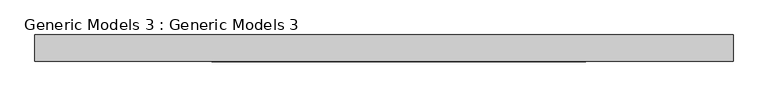
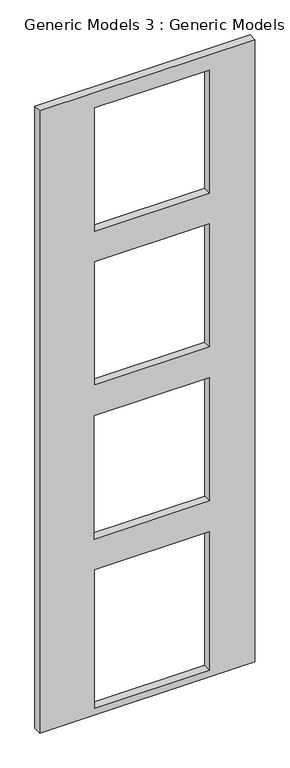
"""IFC4 building model written with IfcOpenShell, lengths in millimetres: proxy geometry, Generic Models 3 : Generic Models 3."""

from ifc_helpers import new_model, si_unit, frame, origin, place, context, project, spatial, polyline, outline, extrude, source, transform, mapped, element, save


def generic_models_3_generic_models_3_7d1dbbdc(model_context):
    return source(origin(), model_context, "Body", "SweptSolid", [
        extrude(outline(polyline([(12192.0, -5583.1675798), (-133.35, -5583.1675798), (-133.35, -1550.9175798), (12192.0, -1550.9175798), (12192.0, -5583.1675798)]), holes=[polyline([(11887.2, -4548.1175798), (11887.2, -2401.8175798), (9448.8, -2401.8175798), (9448.8, -4548.1175798), (11887.2, -4548.1175798)]), polyline([(8839.2, -4548.1175798), (8839.2, -2401.8175798), (6400.8, -2401.8175798), (6400.8, -4548.1175798), (8839.2, -4548.1175798)]), polyline([(5791.2, -4560.8175798), (5791.2, -2401.8175798), (3352.8, -2401.8175798), (3352.8, -4560.8175798), (5791.2, -4560.8175798)]), polyline([(2743.2, -4548.1175798), (2743.2, -2401.8175798), (0.0, -2401.8175798), (0.0, -4548.1175798), (2743.2, -4548.1175798)])]), frame((0.0, -14729.2402089, 0.0), z_axis=(0.0, 1.0, 0.0), x_axis=(0.0, 0.0, 1.0)), (0.0, 0.0, 1.0), 152.4),
    ])


if __name__ == "__main__":
    model = new_model("IFC4")
    model_context = context("Model", 3, world=origin())
    ifc_project = project(units=[si_unit("LENGTHUNIT", "METRE", prefix="MILLI")], contexts=[model_context])
    site = spatial("IfcSite", under=ifc_project)
    building = spatial("IfcBuilding", under=site)
    placement = place(None, origin())
    generic_models_3_generic_models_3_shape = generic_models_3_generic_models_3_7d1dbbdc(model_context)
    element("IfcBuildingElementProxy", 1, Name="Generic Models 3 : Generic Models 3", ObjectType="Generic Models 3 : Generic Models 3", at=placement, inside=building, context=model_context, shape_type="MappedRepresentation", body=[
        mapped(generic_models_3_generic_models_3_shape, transform((0.0, 0.0, 0.0), x_axis=(1.0, 0.0, 0.0), y_axis=(0.0, 1.0, 0.0), z_axis=(0.0, 0.0, 1.0))),
    ])
    save(model, "model.ifc")

# Revit data of these elements
# Element 1 (IfcBuildingElementProxy, "Generic Models 3 : Generic Models 3")
#   Materials on its faces: "brown accent frame"
# Materials
#   "brown accent frame": class "Generic", colour RGB 120 120 120, transparency 0, Cost = 0
